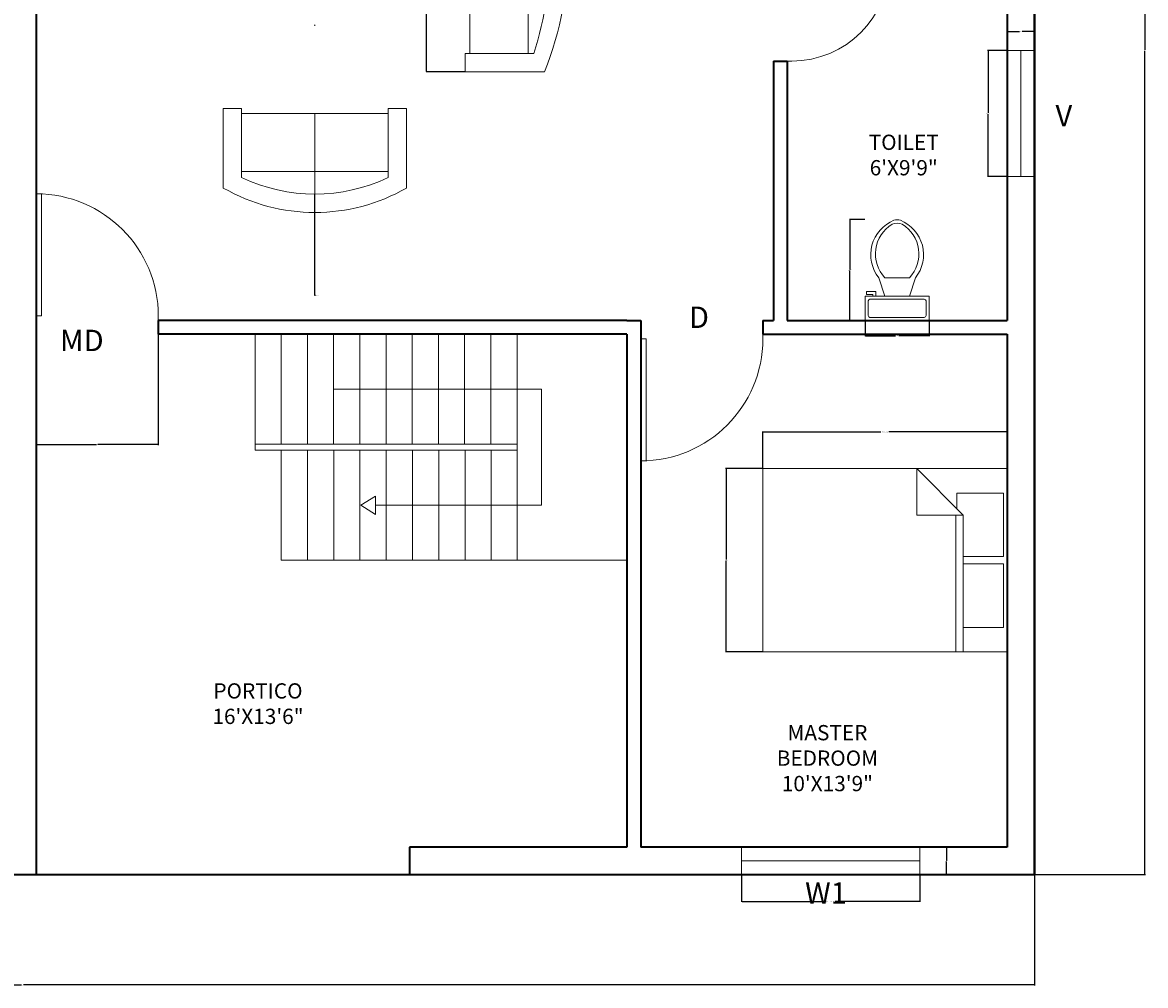
# Model space of a CAD drawing. Units: inches. Extents: x 1939 to 2674, y 558 to 1170.
# Tile 4 of 6: x 2307 to 2674, y 558 to 873. Entities that reach past the tile are written whole.
import ezdxf

# ---------------------------------------------------------------- set-up
doc = ezdxf.new("R2010")
doc.units = ezdxf.units.IN
for name, color, linetype, lineweight in [('A-ANNO-DIMS', 2, 'Continuous', 18), ('A-ANNO-TEXT', 7, 'Continuous', 18), ('A-AREA-IDEN', 7, 'Continuous', 18), ('A-DOOR', 3, 'Continuous', 18), ('A-FLOR-FIXT', 9, 'Continuous', 18), ('A-FLOR-STRS', 7, 'Continuous', 18), ('A-FURN', 8, 'Continuous', 13), ('A-GLAZ', 4, 'Continuous', 18), ('A-WALL', 7, 'Continuous', 35)]:
    doc.layers.add(name, color=color, linetype=linetype, lineweight=lineweight)
doc.styles.get("Standard").update_dxf_attribs({"font": 'arial.ttf'})
doc.dimstyles.get("Standard").update_dxf_attribs({"dimtxt": 0.18, "dimasz": 0.18, "dimexe": 0.18, "dimexo": 0.0625, "dimgap": 0.09, "dimtad": 0, "dimtih": 1, "dimtoh": 1, "dimdec": 4, "dimzin": 0, "dimdsep": 46, "dimtxsty": 'Standard', "dimcen": 0.09, "dimadec": 0, "dimazin": 0, "dimtfac": 1, "dimtdec": 4, "dimtofl": 0, "dimtmove": 0, "dimatfit": 3, "dimfxl": 1, "dimtolj": 1, "dimtzin": 0, "dimarcsym": 0})

# ---------------------------------------------------------------- blocks, each defined once
blk = doc.blocks.new('Sofa - Roundback 7 ft.')
for p, q in [((-12.00002, -32.4421), (-12.00003, -6.5971)), ((11.99997, -32.4421), (11.99998, -6.5971)), ((-36.000027, -34), (-36.000027, -11.4696)), ((-35.999844, -13.3819), (35.9998, -13.3819)), ((35.99998, -34), (35.99998, -11.4696)), ((-36.000027, -32.4421), (35.99998, -32.4421))]:
    blk.add_line(p, q)
for points in [[(-36.000027, -34), (-42.000027, -34), (-42.000027, -8)], [(41.99998, -8), (41.99998, -34), (35.99998, -34)]]:
    blk.add_lwpolyline(points)
for centre, radius, start, end in [((0, -114.25), 114.25, 68.43141, 111.5686), ((-0.00001, -127.1968), 121.1968, 72.72033, 107.2797)]:
    blk.add_arc(centre, radius, start, end)
blk = doc.blocks.new('Toilet - top')
for p, q in [((9.5, -6), (9.5, -2)), ((-10, -8.5), (-8, -8.5)), ((-10, -9.5), (-10, -8.5)), ((-7, -9.5), (-10, -9.5)), ((-8, -8.5), (-8, -8)), ((-7, -8), (-7, -9.5)), ((-4, -8), (-6, -14)), ((4, -8), (6, -14)), ((4, -14), (-4, -14))]:
    blk.add_line(p, q)
blk.add_lwpolyline([(10.5, -8), (10.5, 0), (-10.5, 0), (-10.5, -8)], close=True)
for points in [[(-9.5, -2), (-9.5, -6)], [(8.5, -1), (-8.5, -1)], [(-8.5, -7), (8.5, -7)]]:
    blk.add_lwpolyline(points)
for centre, radius, start, end in [((-8.62, -1.88), 0.884, 81.8699, 188.1301), ((8.62, -1.88), 0.884, 351.8699, 98.1301), ((-8.62, -6.12), 0.884, 171.8699, 278.1301), ((8.62, -6.12), 0.884, 261.8699, 8.1301), ((3.52, -21.58), 12.17, 141.4691, 247.9714), ((4.2, -21.82), 11.33, 136.3677, 238.9468), ((-3.52, -21.58), 12.17, 292.0284, 38.5307), ((-4.2, -21.82), 11.33, 301.053, 43.6321), ((0, -27.88), 4, 245.7318, 294.2682), ((0, -29), 4, 254.8605, 285.1395)]:
    blk.add_arc(centre, radius, start, end)
blk = doc.blocks.new('Bed - Queen')
for p, q in [((0, -80.00003), (0, 0)), ((0, 0), (59.99999, 0)), ((59.99999, 0), (59.99999, -80.00003)), ((7.99999, -1.2), (28.79998, -1.2)), ((7.99999, -14.4), (7.99999, -1.2)), ((28.79998, -1.2), (28.79998, -14.4)), ((31.19999, -1.2), (51.99999, -1.2)), ((31.19999, -14.4), (31.19999, -1.2)), ((51.99999, -1.2), (51.99999, -16.4)), ((0, -14.4), (44.8, -14.4)), ((59.99999, -29.6), (44.8, -14.4)), ((44.8, -14.4), (44.8, -29.6)), ((44.8, -16.8), (0, -16.8)), ((51.99999, -16.4), (46.79936, -16.4)), ((44.8, -29.6), (59.99999, -29.6)), ((59.99999, -80.00003), (0, -80.00003))]:
    blk.add_line(p, q)
blk = doc.blocks.new('Sofa - Roundback Loveseat 5 ft.')
for p, q in [((0, -32.44198), (0, -5.99998)), ((-24, -33.99998), (-24, -11.46958)), ((-23.9998, -13.38178), (23.99986, -13.38178)), ((24.00004, -33.99998), (24.00004, -11.46958)), ((-24, -32.44198), (24.00004, -32.44198))]:
    blk.add_line(p, q)
for points in [[(-24, -33.99998), (-30, -33.99998), (-30, -7.99998)], [(30.00004, -7.99998), (30.00004, -33.99998), (24.00004, -33.99998)]]:
    blk.add_lwpolyline(points)
for centre, radius, start, end in [((0, -60.24998), 60.24998, 60.13715, 119.8628), ((0, -61.38438), 55.38444, 64.32083, 115.6792)]:
    blk.add_arc(centre, radius, start, end)
blk = doc.blocks.new('*U12')
for p, q in [((0, 0), (0, -6)), ((-32, 0), (-32, -6))]:
    blk.add_line(p, q)
blk.add_lwpolyline([(0, 0), (0, 32), (-1.75, 32), (-1.75, 0)], close=True)
blk.add_arc((0, 0), 32, 90, 180)
blk = doc.blocks.new('*U11')
for p, q in [((0, 0), (0, -6)), ((-40, 0), (-40, -6))]:
    blk.add_line(p, q)
blk.add_lwpolyline([(0, 0), (0, 40), (-1.75, 40), (-1.75, 0)], close=True)
blk.add_arc((0, 0), 40, 90, 180)
blk = doc.blocks.new('VENT-TOILET')
for p, q in [((0, 41.35), (9, 41.35)), ((4.5, 0), (4.5, 41.35)), ((0, 0), (9, 0))]:
    blk.add_line(p, q)
blk = doc.blocks.new('WIN-MASTER')
for p, q in [((0, 9), (0, 0)), ((58.35, 9), (58.35, 0)), ((0, 4.5), (58.35, 4.5))]:
    blk.add_line(p, q)
blk = doc.blocks.new('STAIR-RETURN-PORTICO')
for p, q in [((36, 74), (36, 0)), ((44.58, 74), (44.58, 38)), ((53.17, 74), (53.17, 38)), ((61.75, 74), (61.75, 38)), ((70.33, 74), (70.33, 38)), ((78.92, 74), (78.92, 38)), ((87.5, 74), (87.5, 38)), ((96.08, 74), (96.08, 38)), ((104.66, 74), (104.66, 38)), ((113.25, 74), (113.25, 38)), ((121.83, 74), (121.83, 36)), ((96.08, 56), (27.96, 56)), ((27.96, 56), (27.96, 18)), ((36, 38), (121.83, 38)), ((36, 36), (121.83, 36)), ((44.45, 36), (44.45, 0)), ((53.05, 36), (53.05, 0)), ((61.65, 36), (61.65, 0)), ((70.25, 36), (70.25, 0)), ((78.85, 36), (78.85, 0)), ((87.45, 36), (87.45, 0)), ((96.05, 36), (96.05, 0)), ((104.65, 36), (104.65, 0)), ((113.25, 36), (113.25, 0)), ((82.39, 18), (82.39, 21)), ((82.39, 21), (87.13, 18)), ((27.96, 18), (82.39, 18)), ((82.39, 18), (82.39, 15)), ((82.39, 15), (87.13, 18)), ((0, 0), (113.25, 0))]:
    blk.add_line(p, q)
blk = doc.blocks.new('*D20')
at = {"layer": 'A-ANNO-DIMS', "color": 0, "lineweight": -2, "transparency": 16777216}
for p, q in [((2549.05, 727.17), (2549.05, 739.28)), ((2549.23, 739.1), (2587.74, 739.1)), ((2628.87, 739.1), (2590.35, 739.1)), ((2629.05, 727.17), (2629.05, 739.28))]:
    blk.add_line(p, q, dxfattribs=at)
at = {"layer": 'A-ANNO-DIMS', "color": 0, "transparency": 16777216}
for points in [[(2549.23, 739.13), (2549.23, 739.07), (2549.05, 739.1)], [(2628.87, 739.13), (2628.87, 739.07), (2629.05, 739.1)]]:
    blk.add_solid(points, dxfattribs=at)
at = {"layer": 'Defpoints', "color": 0, "transparency": 16777216}
for p in [(2629.05, 739.1), (2549.05, 727.1), (2629.05, 727.1)]:
    blk.add_point(p, dxfattribs=at)
at = {"layer": 'A-ANNO-DIMS', "color": 0, "transparency": 16777216, "insert": (2589.05, 739.1), "char_height": 0.18, "attachment_point": 5}
blk.add_mtext('\\A1;QUEEN BED 80 TYP.', dxfattribs=at)
blk = doc.blocks.new('*D21')
at = {"layer": 'A-ANNO-DIMS', "color": 0, "lineweight": -2, "transparency": 16777216}
for p, q in [((2548.99, 727.1), (2536.87, 727.1)), ((2537.05, 726.92), (2537.05, 697.29)), ((2537.05, 667.28), (2537.05, 696.92)), ((2548.99, 667.1), (2536.87, 667.1))]:
    blk.add_line(p, q, dxfattribs=at)
at = {"layer": 'A-ANNO-DIMS', "color": 0, "transparency": 16777216}
for points in [[(2537.02, 726.92), (2537.08, 726.92), (2537.05, 727.1)], [(2537.02, 667.28), (2537.08, 667.28), (2537.05, 667.1)]]:
    blk.add_solid(points, dxfattribs=at)
at = {"layer": 'Defpoints', "color": 0, "transparency": 16777216}
for p in [(2537.05, 727.1), (2549.05, 727.1), (2549.05, 667.1)]:
    blk.add_point(p, dxfattribs=at)
at = {"layer": 'A-ANNO-DIMS', "color": 0, "transparency": 16777216, "insert": (2537.05, 697.1), "char_height": 0.18, "attachment_point": 5}
blk.add_mtext('\\A1;60 TYP.', dxfattribs=at)
blk = doc.blocks.new('*D26')
at = {"layer": 'A-ANNO-DIMS', "color": 0, "lineweight": -2, "transparency": 16777216}
for p, q in [((2451.46, 941.04), (2438.74, 941.04)), ((2438.92, 940.86), (2438.92, 899.23)), ((2438.92, 857.22), (2438.92, 898.86)), ((2451.46, 857.04), (2438.74, 857.04))]:
    blk.add_line(p, q, dxfattribs=at)
at = {"layer": 'A-ANNO-DIMS', "color": 0, "transparency": 16777216}
for points in [[(2438.89, 940.86), (2438.95, 940.86), (2438.92, 941.04)], [(2438.89, 857.22), (2438.95, 857.22), (2438.92, 857.04)]]:
    blk.add_solid(points, dxfattribs=at)
at = {"layer": 'Defpoints', "color": 0, "transparency": 16777216}
for p in [(2438.92, 941.04), (2451.52, 941.04), (2451.52, 857.04)]:
    blk.add_point(p, dxfattribs=at)
at = {"layer": 'A-ANNO-DIMS', "color": 0, "transparency": 16777216, "insert": (2438.92, 899.04), "char_height": 0.18, "attachment_point": 5}
blk.add_mtext('\\A1;SOFA 84 TYP.', dxfattribs=at)
blk = doc.blocks.new('*D28')
at = {"layer": 'A-ANNO-DIMS', "color": 0, "lineweight": -2, "transparency": 16777216}
for p, q in [((2582.49, 808.66), (2577.41, 808.66)), ((2577.59, 808.48), (2577.59, 792.32)), ((2577.59, 775.79), (2577.59, 791.95)), ((2582.49, 775.61), (2577.41, 775.61))]:
    blk.add_line(p, q, dxfattribs=at)
at = {"layer": 'A-ANNO-DIMS', "color": 0, "transparency": 16777216}
for points in [[(2577.56, 808.48), (2577.62, 808.48), (2577.59, 808.66)], [(2577.56, 775.79), (2577.62, 775.79), (2577.59, 775.61)]]:
    blk.add_solid(points, dxfattribs=at)
at = {"layer": 'Defpoints', "color": 0, "transparency": 16777216}
for p in [(2582.55, 808.66), (2577.59, 775.61), (2582.55, 775.61)]:
    blk.add_point(p, dxfattribs=at)
at = {"layer": 'A-ANNO-DIMS', "color": 0, "transparency": 16777216, "insert": (2577.59, 792.13), "char_height": 0.18, "attachment_point": 5}
blk.add_mtext('\\A1;WC 33 TYP.', dxfattribs=at)
blk = doc.blocks.new('*D29')
at = {"layer": 'A-ANNO-DIMS', "color": 0, "lineweight": -2, "transparency": 16777216}
for p, q in [((2582.55, 775.55), (2582.55, 770.47)), ((2603.55, 775.55), (2603.55, 770.47)), ((2582.73, 770.65), (2592.52, 770.65)), ((2603.37, 770.65), (2593.58, 770.65))]:
    blk.add_line(p, q, dxfattribs=at)
at = {"layer": 'A-ANNO-DIMS', "color": 0, "transparency": 16777216}
for points in [[(2582.73, 770.68), (2582.73, 770.62), (2582.55, 770.65)], [(2603.37, 770.68), (2603.37, 770.62), (2603.55, 770.65)]]:
    blk.add_solid(points, dxfattribs=at)
at = {"layer": 'Defpoints', "color": 0, "transparency": 16777216}
for p in [(2582.55, 775.61), (2603.55, 775.61), (2603.55, 770.65)]:
    blk.add_point(p, dxfattribs=at)
at = {"layer": 'A-ANNO-DIMS', "color": 0, "transparency": 16777216, "insert": (2593.05, 770.65), "char_height": 0.18, "attachment_point": 5}
blk.add_mtext('\\A1;21 TYP.', dxfattribs=at)
blk = doc.blocks.new('*D44')
at = {"layer": 'A-ANNO-DIMS', "color": 0, "lineweight": -2, "transparency": 16777216}
for p, q in [((2628.99, 864.11), (2622.67, 864.11)), ((2622.85, 863.93), (2622.85, 843.62)), ((2622.85, 822.94), (2622.85, 843.26)), ((2628.99, 822.76), (2622.67, 822.76))]:
    blk.add_line(p, q, dxfattribs=at)
at = {"layer": 'A-ANNO-DIMS', "color": 0, "transparency": 16777216}
for points in [[(2622.82, 863.93), (2622.88, 863.93), (2622.85, 864.11)], [(2622.82, 822.94), (2622.88, 822.94), (2622.85, 822.76)]]:
    blk.add_solid(points, dxfattribs=at)
at = {"layer": 'Defpoints', "color": 0, "transparency": 16777216}
for p in [(2629.05, 864.11), (2622.85, 822.76), (2629.05, 822.76)]:
    blk.add_point(p, dxfattribs=at)
at = {"layer": 'A-ANNO-DIMS', "color": 0, "transparency": 16777216, "insert": (2622.85, 843.44), "char_height": 0.18, "attachment_point": 5}
blk.add_mtext('\\A1;VENT 41 TYP.', dxfattribs=at)
blk = doc.blocks.new('*D45')
at = {"layer": 'A-ANNO-DIMS', "color": 0, "lineweight": -2, "transparency": 16777216}
for p, q in [((2629.05, 864.17), (2629.05, 870.49)), ((2629.23, 870.31), (2633.09, 870.31)), ((2637.87, 870.31), (2634.01, 870.31)), ((2638.05, 864.17), (2638.05, 870.49))]:
    blk.add_line(p, q, dxfattribs=at)
at = {"layer": 'A-ANNO-DIMS', "color": 0, "transparency": 16777216}
for points in [[(2629.23, 870.34), (2629.23, 870.28), (2629.05, 870.31)], [(2637.87, 870.34), (2637.87, 870.28), (2638.05, 870.31)]]:
    blk.add_solid(points, dxfattribs=at)
at = {"layer": 'Defpoints', "color": 0, "transparency": 16777216}
for p in [(2629.05, 870.31), (2629.05, 864.11), (2638.05, 864.11)]:
    blk.add_point(p, dxfattribs=at)
at = {"layer": 'A-ANNO-DIMS', "color": 0, "transparency": 16777216, "insert": (2633.55, 870.31), "char_height": 0.18, "attachment_point": 5}
blk.add_mtext('\\A1;9 TYP.', dxfattribs=at)
blk = doc.blocks.new('*D46')
at = {"layer": 'A-ANNO-DIMS', "color": 0, "lineweight": -2, "transparency": 16777216}
for p, q in [((2542.08, 594.05), (2542.08, 585.18)), ((2600.43, 594.05), (2600.43, 585.18)), ((2542.26, 585.36), (2569.81, 585.36)), ((2600.25, 585.36), (2572.7, 585.36))]:
    blk.add_line(p, q, dxfattribs=at)
at = {"layer": 'A-ANNO-DIMS', "color": 0, "transparency": 16777216}
for points in [[(2542.26, 585.39), (2542.26, 585.33), (2542.08, 585.36)], [(2600.25, 585.39), (2600.25, 585.33), (2600.43, 585.36)]]:
    blk.add_solid(points, dxfattribs=at)
at = {"layer": 'Defpoints', "color": 0, "transparency": 16777216}
for p in [(2542.08, 594.11), (2600.43, 594.11), (2600.43, 585.36)]:
    blk.add_point(p, dxfattribs=at)
at = {"layer": 'A-ANNO-DIMS', "color": 0, "transparency": 16777216, "insert": (2571.26, 585.36), "char_height": 0.18, "attachment_point": 5}
blk.add_mtext('\\A1;MASTER WDW 58 TYP.', dxfattribs=at)
blk = doc.blocks.new('*D47')
at = {"layer": 'A-ANNO-DIMS', "color": 0, "lineweight": -2, "transparency": 16777216}
for p, q in [((2600.49, 603.11), (2609.36, 603.11)), ((2609.18, 602.93), (2609.18, 598.79)), ((2609.18, 594.29), (2609.18, 598.43)), ((2600.49, 594.11), (2609.36, 594.11))]:
    blk.add_line(p, q, dxfattribs=at)
at = {"layer": 'A-ANNO-DIMS', "color": 0, "transparency": 16777216}
for points in [[(2609.15, 602.93), (2609.21, 602.93), (2609.18, 603.11)], [(2609.15, 594.29), (2609.21, 594.29), (2609.18, 594.11)]]:
    blk.add_solid(points, dxfattribs=at)
at = {"layer": 'Defpoints', "color": 0, "transparency": 16777216}
for p in [(2600.43, 603.11), (2609.18, 603.11), (2600.43, 594.11)]:
    blk.add_point(p, dxfattribs=at)
at = {"layer": 'A-ANNO-DIMS', "color": 0, "transparency": 16777216, "insert": (2609.18, 598.61), "char_height": 0.18, "attachment_point": 5}
blk.add_mtext('\\A1;9 TYP.', dxfattribs=at)
blk = doc.blocks.new('*D50')
at = {"layer": 'A-ANNO-DIMS', "color": 0, "lineweight": -2, "transparency": 16777216}
for p, q in [((2638.11, 1134.11), (2674.38, 1134.11)), ((2674.2, 1133.93), (2674.2, 864.29)), ((2674.2, 594.29), (2674.2, 863.93)), ((2638.11, 594.11), (2674.38, 594.11))]:
    blk.add_line(p, q, dxfattribs=at)
at = {"layer": 'A-ANNO-DIMS', "color": 0, "transparency": 16777216}
for points in [[(2674.17, 1133.93), (2674.23, 1133.93), (2674.2, 1134.11)], [(2674.17, 594.29), (2674.23, 594.29), (2674.2, 594.11)]]:
    blk.add_solid(points, dxfattribs=at)
at = {"layer": 'Defpoints', "color": 0, "transparency": 16777216}
for p in [(2638.05, 1134.11), (2674.2, 1134.11), (2638.05, 594.11)]:
    blk.add_point(p, dxfattribs=at)
at = {"layer": 'A-ANNO-DIMS', "color": 0, "transparency": 16777216, "insert": (2674.2, 864.11), "char_height": 0.18, "attachment_point": 5}
blk.add_mtext('\\A1;540', dxfattribs=at)
blk = doc.blocks.new('*D51')
at = {"layer": 'A-ANNO-DIMS', "color": 0, "lineweight": -2, "transparency": 16777216}
for p, q in [((1975.05, 594.05), (1975.05, 557.78)), ((2638.05, 594.05), (2638.05, 557.78)), ((1975.23, 557.96), (2306.26, 557.96)), ((2637.87, 557.96), (2306.84, 557.96))]:
    blk.add_line(p, q, dxfattribs=at)
at = {"layer": 'A-ANNO-DIMS', "color": 0, "transparency": 16777216}
for points in [[(1975.23, 557.99), (1975.23, 557.93), (1975.05, 557.96)], [(2637.87, 557.99), (2637.87, 557.93), (2638.05, 557.96)]]:
    blk.add_solid(points, dxfattribs=at)
at = {"layer": 'Defpoints', "color": 0, "transparency": 16777216}
for p in [(1975.05, 594.11), (2638.05, 594.11), (2638.05, 557.96)]:
    blk.add_point(p, dxfattribs=at)
at = {"layer": 'A-ANNO-DIMS', "color": 0, "transparency": 16777216, "insert": (2306.55, 557.96), "char_height": 0.18, "attachment_point": 5}
blk.add_mtext('\\A1;663', dxfattribs=at)
blk = doc.blocks.new('*D52')
at = {"layer": 'A-ANNO-DIMS', "color": 0, "lineweight": -2, "transparency": 16777216}
for p, q in [((2311.05, 771.05), (2311.05, 734.78)), ((2351.05, 771.05), (2351.05, 734.78)), ((2311.23, 734.96), (2330.83, 734.96)), ((2350.87, 734.96), (2331.27, 734.96))]:
    blk.add_line(p, q, dxfattribs=at)
at = {"layer": 'A-ANNO-DIMS', "color": 0, "transparency": 16777216}
for points in [[(2311.23, 734.99), (2311.23, 734.93), (2311.05, 734.96)], [(2350.87, 734.99), (2350.87, 734.93), (2351.05, 734.96)]]:
    blk.add_solid(points, dxfattribs=at)
at = {"layer": 'Defpoints', "color": 0, "transparency": 16777216}
for p in [(2311.05, 771.11), (2351.05, 771.11), (2311.05, 734.96)]:
    blk.add_point(p, dxfattribs=at)
at = {"layer": 'A-ANNO-DIMS', "color": 0, "transparency": 16777216, "insert": (2331.05, 734.96), "char_height": 0.18, "attachment_point": 5}
blk.add_mtext('\\A1;40', dxfattribs=at)
blk = doc.blocks.new('*D76')
at = {"layer": 'A-ANNO-DIMS', "color": 0, "lineweight": -2, "transparency": 16777216}
for p, q in [((2402.25, 872.4), (2402.43, 872.4)), ((2402.34, 872.31), (2402.34, 872.49)), ((2402.34, 783.78), (2402.34, 816.84)), ((2402.52, 783.78), (2402.34, 783.78))]:
    blk.add_line(p, q, dxfattribs=at)
at = {"layer": 'A-ANNO-DIMS', "color": 0, "transparency": 16777216}
blk.add_solid([(2402.37, 816.84), (2402.31, 816.84), (2402.34, 817.02)], dxfattribs=at)
at = {"layer": 'Defpoints', "color": 0, "transparency": 16777216}
for p in [(2402.34, 872.4), (2402.34, 817.02)]:
    blk.add_point(p, dxfattribs=at)
at = {"layer": 'A-ANNO-DIMS', "color": 0, "transparency": 16777216, "insert": (2403.2, 783.78), "char_height": 0.18, "attachment_point": 5}
blk.add_mtext('\\A1;4X R55.38', dxfattribs=at)

msp = doc.modelspace()

# ---------------------------------------------------------------- linework, layer by layer
at = {"layer": 'A-WALL'}
for p, q in [((2638.048, 594.1102), (2638.048, 1134.1102)), ((2638.048, 1134.1102), (2638.048, 594.1102)), ((2311.048, 1017.1102), (2311.048, 771.1102)), ((2629.048, 892.6102), (2629.048, 775.6102)), ((2552.548, 860.6102), (2552.548, 775.6102)), ((2552.548, 860.6102), (2557.048, 860.6102)), ((2557.048, 860.6102), (2557.048, 775.6102)), ((2504.548, 775.6102), (2351.048, 775.6102)), ((2351.048, 775.6102), (2351.048, 771.1102)), ((2351.048, 775.6102), (2351.048, 771.1102)), ((2504.548, 775.6102), (2509.048, 775.6102)), ((2509.048, 775.6102), (2509.048, 603.1102)), ((2549.048, 775.6102), (2552.548, 775.6102)), ((2549.048, 775.6102), (2549.048, 771.1102)), ((2557.048, 775.6102), (2629.048, 775.6102)), ((2311.048, 771.1102), (2311.048, 594.1102)), ((2504.548, 771.1102), (2351.048, 771.1102)), ((2504.548, 771.1102), (2504.548, 603.1102)), ((2549.048, 771.1102), (2629.048, 771.1102)), ((2629.048, 771.1102), (2629.048, 603.1102)), ((2504.548, 603.1102), (2433.3071, 603.1102)), ((2433.3071, 603.1102), (2433.3071, 594.1102)), ((2629.048, 603.1102), (2509.048, 603.1102)), ((1975.0479, 594.1102), (2638.048, 594.1102))]:
    msp.add_line(p, q, dxfattribs=at)

# ---------------------------------------------------------------- block references
at = {"layer": 'A-DOOR', "xscale": -1, "rotation": 270}
msp.add_blockref('*U12', (2558.548, 892.6102), dxfattribs=at)
at = {"layer": 'A-DOOR', "xscale": -1}
msp.add_blockref('*U11', (2311.048, 777.1102), dxfattribs=at)
at = {"layer": 'A-DOOR', "rotation": 180}
msp.add_blockref('*U11', (2509.048, 769.6102), dxfattribs=at)
at = {"layer": 'A-FLOR-FIXT', "xscale": -1, "rotation": 180}
msp.add_blockref('Toilet - top', (2593.048, 775.6102), dxfattribs=at)
at = {"layer": 'A-FLOR-STRS', "extrusion": (0, 0, -1), "zscale": -1}
msp.add_blockref('STAIR-RETURN-PORTICO', (-2504.548, 697.1102), dxfattribs=at)
at = {"layer": 'A-FURN', "xscale": -1, "rotation": 270}
for name, p in [('Sofa - Roundback 7 ft.', (2485.525, 899.043)), ('Bed - Queen', (2629.048, 667.1037))]:
    msp.add_blockref(name, p, dxfattribs=at)
at = {"layer": 'A-FURN', "rotation": 180}
msp.add_blockref('Sofa - Roundback Loveseat 5 ft.', (2402.3387, 811.0152), dxfattribs=at)
at = {"layer": 'A-GLAZ', "rotation": 180}
msp.add_blockref('VENT-TOILET', (2638.048, 864.1102), dxfattribs=at)
at = {"layer": 'A-GLAZ'}
msp.add_blockref('WIN-MASTER', (2542.0813, 594.1102), dxfattribs=at)

# ---------------------------------------------------------------- texts
at = {"layer": 'A-ANNO-TEXT', "char_height": 7, "attachment_point": 3}
for s, insert in [('\\pxqc;V', (2658.5924, 846.2453)), ('\\pxqc;D', (2539.0649, 780.1743)), ('\\pxqc;MD', (2336.9338, 772.5911)), ('\\pxqc;W1', (2580.6858, 591.5736))]:
    msp.add_mtext_dynamic_manual_height_columns(s, width=21.893501, gutter_width=12.5, heights=[0], dxfattribs=dict(at, insert=insert))
at = {"layer": 'A-AREA-IDEN', "char_height": 5, "attachment_point": 3}
for s, insert in [('\\pxqc;TOILET\\P6\'X9\'9"', (2614.7585, 836.4962)), ('\\pxqc;PORTICO\\P16\'X13\'6"', (2403.2481, 656.7886)), ('\\pxqc;MASTER\\PBEDROOM\\P10\'X13\'9"', (2589.7572, 643.1082))]:
    msp.add_mtext_dynamic_manual_height_columns(s, width=39.116177, gutter_width=12.5, heights=[0], dxfattribs=dict(at, insert=insert))

# ---------------------------------------------------------------- dimensions: what is measured, and where the dimension line sits
at = {"layer": 'A-ANNO-DIMS'}
for base, p1, p2, angle, picture, middle in [((2674.198, 1134.1102), (2638.048, 594.1102), (2638.048, 1134.1102), 90, '*D50', (2674.198, 864.1102)), ((2311.048, 734.9602), (2351.048, 771.1102), (2311.048, 771.1102), 180, '*D52', (2331.048, 734.9602))]:
    dim = msp.add_linear_dim(base=base, p1=p1, p2=p2, angle=angle, dimstyle='Standard', override={"dimdec": 0, "dimlfac": 1, "dimrnd": 0, "dimzin": 0, "dimdsep": 46, "dimlunit": 2}, dxfattribs=at)
    dim.commit()
    dim.dimension.update_dxf_attribs({"geometry": picture, "text_midpoint": middle})
for base, p1, p2, angle, text, picture, middle in [((2438.925, 941.043), (2451.525, 857.0429), (2451.525, 941.043), 90, 'SOFA <> TYP.', '*D26', (2438.925, 899.0429)), ((2629.048, 870.3126), (2638.048, 864.1102), (2629.048, 864.1102), 180, '<> TYP.', '*D45', (2633.548, 870.3126)), ((2622.8456, 822.7612), (2629.048, 864.1102), (2629.048, 822.7612), 270, 'VENT <> TYP.', '*D44', (2622.8456, 843.4357)), ((2577.591, 775.6102), (2582.548, 808.6565), (2582.548, 775.6102), 270, 'WC <> TYP.', '*D28', (2577.591, 792.1333)), ((2537.0479, 727.1037), (2549.0479, 667.1037), (2549.0479, 727.1037), 90, '<> TYP.', '*D21', (2537.0479, 697.1037)), ((2609.1844, 603.1102), (2600.4318, 594.1102), (2600.4318, 603.1102), 90, '<> TYP.', '*D47', (2609.1844, 598.6102))]:
    dim = msp.add_linear_dim(base=base, p1=p1, p2=p2, angle=angle, text=text, dimstyle='Standard', override={"dimdec": 0, "dimlfac": 1, "dimrnd": 0, "dimzin": 0, "dimdsep": 46, "dimlunit": 2}, dxfattribs=at)
    dim.commit()
    dim.dimension.update_dxf_attribs({"geometry": picture, "text_midpoint": middle})
dim = msp.add_radius_dim(center=(2402.3387, 872.3996), mpoint=(2402.339, 817.0152), text='4X <>', dimstyle='Standard', override={"dimdec": 2, "dimlfac": 1, "dimrnd": 0, "dimzin": 0, "dimdsep": 46, "dimlunit": 2}, dxfattribs=at)
dim.commit()
dim.dimension.update_dxf_attribs({"geometry": '*D76', "text_midpoint": (2403.1962, 783.7845), "dimtype": 164})
for base, p1, p2, text, picture, middle in [((2603.548, 770.6533), (2582.548, 775.6102), (2603.548, 775.6102), '<> TYP.', '*D29', (2593.048, 770.6533)), ((2629.048, 739.1037), (2549.0479, 727.1037), (2629.048, 727.1037), 'QUEEN BED <> TYP.', '*D20', (2589.0479, 739.1037)), ((2600.4318, 585.3576), (2542.0813, 594.1102), (2600.4318, 594.1102), 'MASTER WDW <> TYP.', '*D46', (2571.2565, 585.3576))]:
    dim = msp.add_linear_dim(base=base, p1=p1, p2=p2, text=text, dimstyle='Standard', override={"dimdec": 0, "dimlfac": 1, "dimrnd": 0, "dimzin": 0, "dimdsep": 46, "dimlunit": 2}, dxfattribs=at)
    dim.commit()
    dim.dimension.update_dxf_attribs({"geometry": picture, "text_midpoint": middle})
dim = msp.add_linear_dim(base=(2638.048, 557.9602), p1=(1975.0479, 594.1102), p2=(2638.048, 594.1102), dimstyle='Standard', override={"dimdec": 0, "dimlfac": 1, "dimrnd": 0, "dimzin": 0, "dimdsep": 46, "dimlunit": 2}, dxfattribs=at)
dim.commit()
dim.dimension.update_dxf_attribs({"geometry": '*D51', "text_midpoint": (2306.548, 557.9602)})

doc.saveas('drawing.dxf')
